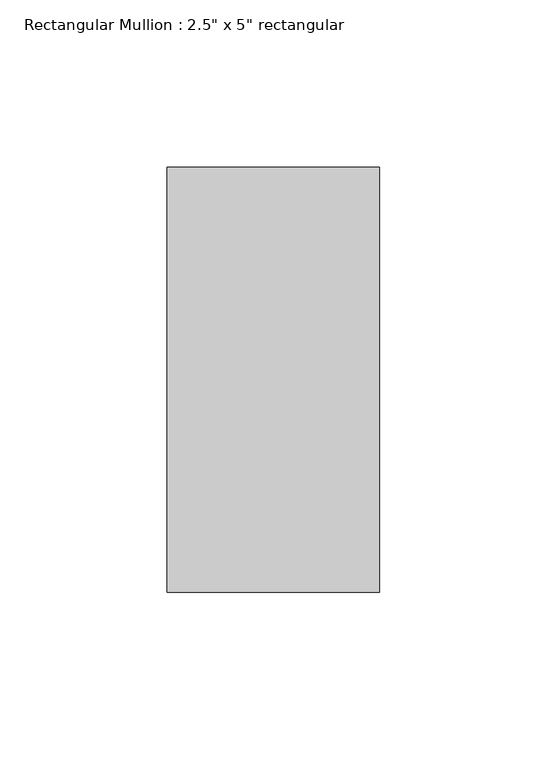
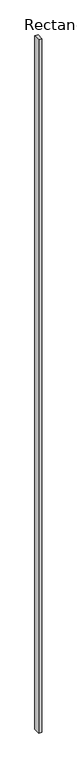
"""IFC4 building model written with IfcOpenShell, lengths in millimetres: member geometry."""

from ifc_helpers import new_model, si_unit, frame, origin, place, context, project, spatial, polyline, outline, extrude, source, transform, mapped, element, save


def member_d26f5695(model_context):
    return source(origin(), model_context, "Body", "SweptSolid", [
        extrude(outline(polyline([(31.75, 63.5), (31.75, -63.5), (-31.75, -63.5), (-31.75, 63.5), (31.75, 63.5)])), frame((0.0, 0.0, -14630.4), z_axis=(0.0, 0.0, 1.0), x_axis=(1.0, 0.0, 0.0)), (0.0, 0.0, 1.0), 14630.4),
    ])


if __name__ == "__main__":
    model = new_model("IFC4")
    model_context = context("Model", 3, world=origin())
    ifc_project = project(units=[si_unit("LENGTHUNIT", "METRE", prefix="MILLI")], contexts=[model_context])
    site = spatial("IfcSite", under=ifc_project)
    building = spatial("IfcBuilding", under=site)
    placement = place(None, origin())
    member_shape = member_d26f5695(model_context)
    element("IfcMember", 1, ObjectType="Rectangular Mullion : 2.5\" x 5\" rectangular", at=placement, inside=building, context=model_context, shape_type="MappedRepresentation", body=[
        mapped(member_shape, transform((0.0, 0.0, 0.0), x_axis=(1.0, 0.0, 0.0), y_axis=(0.0, 1.0, 0.0), z_axis=(0.0, 0.0, 1.0))),
    ])
    save(model, "model.ifc")

# Revit data of these elements
# Type "Rectangular Mullion : 2.5\" x 5\" rectangular"
#   built-in parameter 1007304 = 0.416667 (stored number, unit not read)
#   built-in parameter 1007301 = 0.104167 (stored number, unit not read)
#   built-in parameter 1007300 = 0.104167 (stored number, unit not read)
# Element 1 (IfcMember, "Rectangular Mullion : 2.5\" x 5\" rectangular")
#   Materials on its faces: "Aluminum"
# Materials
#   "Aluminum": class "Metal", colour RGB 247 247 247, transparency 0, Description = "Aluminum 6061", Cost = 0
